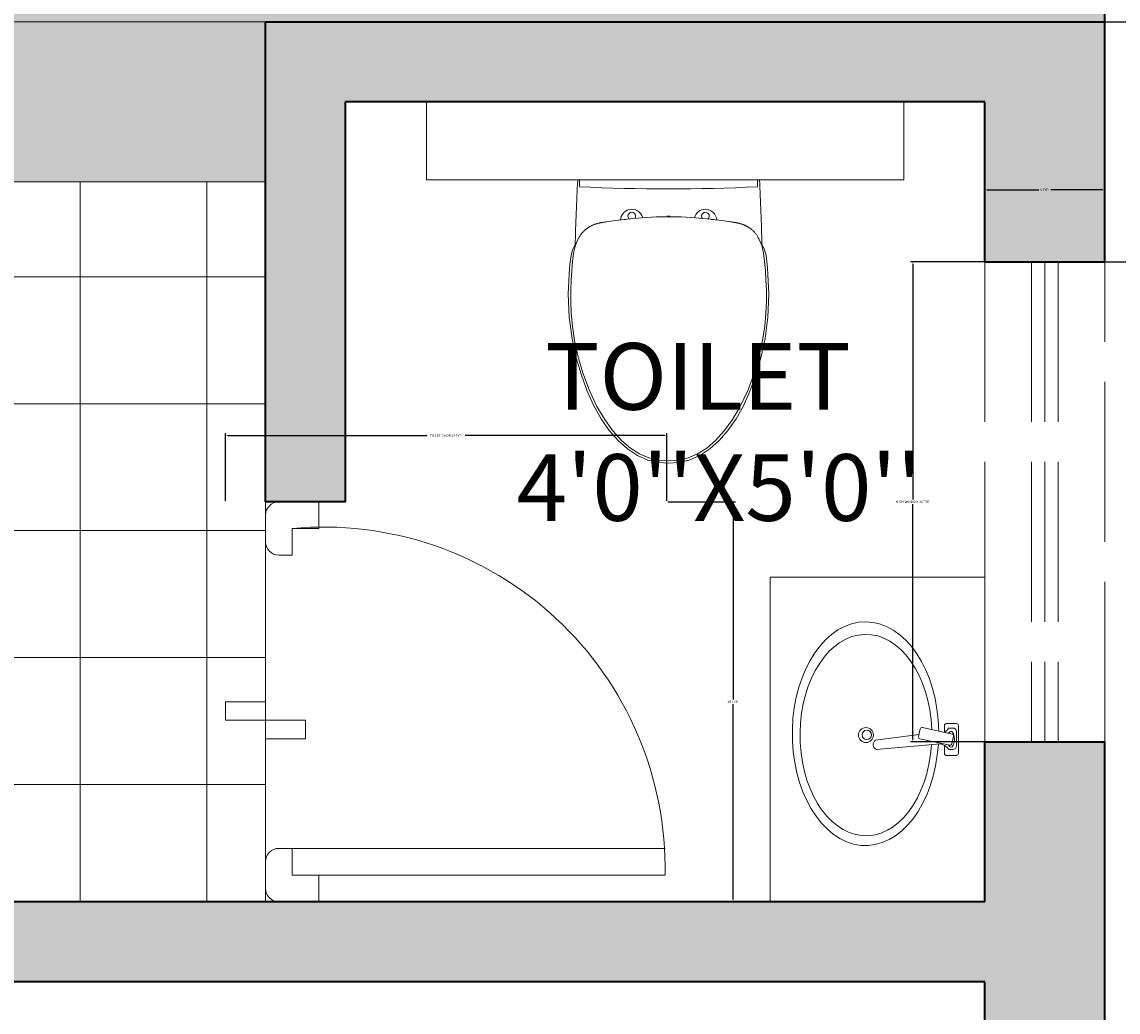
# Model space of a CAD drawing. Units: inches. Extents: x 84 to 1044, y -280 to 906.
# Tile 80 of 105: x 815 to 897, y 326 to 400. Entities that reach past the tile are written whole.
import ezdxf

# ---------------------------------------------------------------- set-up
doc = ezdxf.new("R2010")
doc.units = ezdxf.units.IN
doc.linetypes.add('ACAD_ISO02W100', pattern=[15, 12, -3])
for name, color, linetype, lineweight in [('00 FURNITURE', 15, 'Continuous', 15), ('A-ANNO-DIMS', 2, 'Continuous', 18), ('A-AREA-IDEN', 7, 'Continuous', 13), ('A-DOOR', 4, 'Continuous', 18), ('A-FLOR-FIXT', 9, 'Continuous', 15), ('A-GLAZ-HIGH', 160, 'ACAD_ISO02W100', 13), ('A-STAIRCASE', 144, 'Continuous', 18), ('A_FUR 1', 5, 'Continuous', 5), ('WALL', 250, 'Continuous', 35)]:
    doc.layers.add(name, color=color, linetype=linetype, lineweight=lineweight)
for name, color, linetype, lineweight, true_color in [('A-FLOR-PATT', 251, 'Continuous', 9, 0x705861), ('A-FLOR-STRS-PATT', 35, 'Continuous', 9, 0x947764), ('A-WALL-PATT', 251, 'Continuous', 9, 0x636466), ('L-PLNT-PATT', 9, 'Continuous', 9, 0xafd9aa)]:
    doc.layers.add(name, color=color, linetype=linetype, lineweight=lineweight, true_color=true_color)
doc.styles.add('1-100DIM', font='txt', dxfattribs={"height": 0.3})
doc.styles.get("Standard").update_dxf_attribs({"font": 'arial.ttf'})
doc.dimstyles.get("Standard").update_dxf_attribs({"dimtxt": 0.18, "dimasz": 0.18, "dimexe": 0.18, "dimexo": 0.0625, "dimgap": 0.09, "dimtad": 0, "dimtih": 1, "dimtoh": 1, "dimdec": 4, "dimzin": 0, "dimdsep": 46, "dimtxsty": 'Standard', "dimcen": 0.09, "dimadec": 0, "dimazin": 0, "dimtfac": 1, "dimtdec": 4, "dimtofl": 0, "dimtmove": 0, "dimatfit": 3, "dimfxl": 1, "dimtolj": 1, "dimtzin": 0, "dimarcsym": 0})

# ---------------------------------------------------------------- blocks, each defined once
blk = doc.blocks.new('ESTSET')
at = {"layer": 'A_FUR 1'}
for p, q in [((-10.444, 4.097), (-10.444, 32.097)), ((-8.444, 4.097), (-8.444, 32.097)), ((-36.444, 6.097), (-36.444, 3.097)), ((-34.444, 6.097), (-36.444, 6.097)), ((-34.444, 4.097), (-34.444, 6.097)), ((-34.444, 4.097), (-34.444, 6.097)), ((-8.444, 4.097), (-8.444, 6.097)), ((-8.444, 6.097), (-6.444, 6.097)), ((-8.444, 4.097), (-8.444, 6.097)), ((-6.444, 6.097), (-6.444, 3.097)), ((-32.444, 4.097), (-34.444, 4.097)), ((-32.444, 4.097), (-34.444, 4.097)), ((-32.444, 3.097), (-32.444, 4.097)), ((-10.444, 3.097), (-10.444, 4.097)), ((-10.444, 4.097), (-8.444, 4.097)), ((-10.444, 4.097), (-8.444, 4.097)), ((-6.444, 2.097), (-36.444, 2.097)), ((-35.444, 2.097), (-33.444, 2.097)), ((-7.444, 2.097), (-9.444, 2.097))]:
    blk.add_line(p, q, dxfattribs=at)
for points in [[(-21.444, 2.097), (-18.672, 2.097), (-18.672, 5.102), (-20.058, 5.102)], [(-20.058, 5.102), (-20.058, -0.909)], [(-21.444, 2.097), (-21.444, -0.909), (-20.058, -0.909)]]:
    blk.add_lwpolyline(points, dxfattribs=at)
for centre, radius, start, end in [((-8.909, 6.457), 25.644, 88.96059, 185.2816), ((-35.444, 3.097), 1, 180, 270), ((-33.444, 3.097), 1, 270, 0), ((-9.444, 3.097), 1, 180, 270), ((-7.444, 3.097), 1, 270, 0)]:
    blk.add_arc(centre, radius, start, end, dxfattribs=at)
blk = doc.blocks.new('32')
at = {"layer": '00 FURNITURE'}
for p, q in [((-6.823, 0), (6.823, 0)), ((-6.685, -0.511), (-6.685, 0)), ((6.237, 0), (6.685, 0)), ((6.685, -0.511), (6.685, 0)), ((-5.414, -3.288), (-5.444, -3.297)), ((-5.385, -3.279), (-5.414, -3.288)), ((-5.356, -3.271), (-5.385, -3.279)), ((-5.328, -3.264), (-5.356, -3.271)), ((-5.301, -3.256), (-5.328, -3.264)), ((-5.273, -3.249), (-5.301, -3.256)), ((-5.247, -3.242), (-5.273, -3.249)), ((-5.22, -3.236), (-5.247, -3.242)), ((-5.195, -3.23), (-5.22, -3.236)), ((-5.17, -3.225), (-5.195, -3.23)), ((-5.145, -3.219), (-5.17, -3.225)), ((-5.121, -3.214), (-5.145, -3.219)), ((-5.098, -3.209), (-5.121, -3.214)), ((-5.076, -3.205), (-5.098, -3.209)), ((-5.053, -3.2), (-5.076, -3.205)), ((-5.032, -3.196), (-5.053, -3.2)), ((-5.011, -3.193), (-5.032, -3.196)), ((-4.97, -3.185), (-5.011, -3.193)), ((-4.931, -3.179), (-4.97, -3.185)), ((-4.893, -3.173), (-4.931, -3.179)), ((-4.858, -3.167), (-4.893, -3.173)), ((-4.824, -3.162), (-4.858, -3.167)), ((-4.776, -3.155), (-4.824, -3.162)), ((-4.717, -3.147), (-4.776, -3.155)), ((-4.627, -3.135), (-4.717, -3.147)), ((-4.464, -3.111), (-4.637, -3.136)), ((-4.345, -3.095), (-4.464, -3.111)), ((-4.151, -3.069), (-4.345, -3.095)), ((-3.99, -3.048), (-4.151, -3.069)), ((-3.77, -3.021), (-3.99, -3.048)), ((-3.503, -2.989), (-3.77, -3.021)), ((-3.335, -2.969), (-3.503, -2.989)), ((-3.3, -2.966), (-3.32, -2.968)), ((-3.257, -2.962), (-3.3, -2.966)), ((-3.212, -2.958), (-3.257, -2.962)), ((-3.146, -2.951), (-3.205, -2.957)), ((-2.011, -2.841), (-3.146, -2.951)), ((-0.935, -2.777), (-2.011, -2.841)), ((0, -2.757), (-0.935, -2.777)), ((0.118, -2.713), (-0.118, -2.713)), ((0, -2.757), (0.935, -2.777)), ((0.935, -2.777), (2.011, -2.841)), ((2.011, -2.841), (3.146, -2.951)), ((3.146, -2.951), (3.205, -2.957)), ((3.212, -2.958), (3.257, -2.962)), ((3.257, -2.962), (3.3, -2.966)), ((3.3, -2.966), (3.32, -2.968)), ((3.335, -2.969), (3.503, -2.989)), ((3.503, -2.989), (3.77, -3.021)), ((3.77, -3.021), (3.99, -3.048)), ((3.99, -3.048), (4.151, -3.069)), ((4.151, -3.069), (4.345, -3.095)), ((4.345, -3.095), (4.464, -3.111)), ((4.464, -3.111), (4.637, -3.136)), ((4.627, -3.135), (4.717, -3.147)), ((4.717, -3.147), (4.776, -3.155)), ((4.776, -3.155), (4.824, -3.162)), ((4.824, -3.162), (4.858, -3.167)), ((4.858, -3.167), (4.893, -3.173)), ((4.893, -3.173), (4.931, -3.179)), ((4.931, -3.179), (4.97, -3.185)), ((4.97, -3.185), (5.011, -3.193)), ((5.011, -3.193), (5.032, -3.196)), ((5.032, -3.196), (5.053, -3.2)), ((5.053, -3.2), (5.076, -3.205)), ((5.076, -3.205), (5.098, -3.209)), ((5.098, -3.209), (5.121, -3.214)), ((5.121, -3.214), (5.145, -3.219)), ((5.145, -3.219), (5.17, -3.225)), ((5.17, -3.225), (5.195, -3.23)), ((5.195, -3.23), (5.22, -3.236)), ((5.22, -3.236), (5.247, -3.242)), ((5.247, -3.242), (5.273, -3.249)), ((5.273, -3.249), (5.301, -3.256)), ((5.301, -3.256), (5.328, -3.264)), ((5.328, -3.264), (5.356, -3.271)), ((5.356, -3.271), (5.385, -3.279)), ((5.385, -3.279), (5.414, -3.288)), ((5.414, -3.288), (5.444, -3.297)), ((-6.579, -4.082), (-6.611, -4.127)), ((-6.547, -4.039), (-6.579, -4.082)), ((-6.514, -3.997), (-6.547, -4.039)), ((-6.481, -3.958), (-6.514, -3.997)), ((-6.447, -3.92), (-6.481, -3.958)), ((-6.413, -3.882), (-6.447, -3.92)), ((-6.378, -3.847), (-6.413, -3.882)), ((-6.343, -3.813), (-6.378, -3.847)), ((-6.307, -3.779), (-6.343, -3.813)), ((-6.271, -3.748), (-6.307, -3.779)), ((-6.235, -3.717), (-6.271, -3.748)), ((-6.199, -3.687), (-6.235, -3.717)), ((-6.162, -3.659), (-6.199, -3.687)), ((-6.125, -3.632), (-6.162, -3.659)), ((-6.088, -3.606), (-6.125, -3.632)), ((-6.052, -3.581), (-6.088, -3.606)), ((-6.015, -3.557), (-6.052, -3.581)), ((-5.978, -3.535), (-6.015, -3.557)), ((-5.942, -3.513), (-5.978, -3.535)), ((-5.906, -3.493), (-5.942, -3.513)), ((-5.869, -3.473), (-5.906, -3.493)), ((-5.834, -3.455), (-5.869, -3.473)), ((-5.798, -3.437), (-5.834, -3.455)), ((-5.763, -3.421), (-5.798, -3.437)), ((-5.729, -3.405), (-5.763, -3.421)), ((-5.695, -3.39), (-5.729, -3.405)), ((-5.662, -3.376), (-5.695, -3.39)), ((-5.629, -3.363), (-5.662, -3.376)), ((-5.597, -3.351), (-5.629, -3.363)), ((-5.565, -3.339), (-5.597, -3.351)), ((-5.534, -3.328), (-5.565, -3.339)), ((-5.504, -3.317), (-5.534, -3.328)), ((-5.474, -3.307), (-5.504, -3.317)), ((-5.444, -3.297), (-5.474, -3.307)), ((5.444, -3.297), (5.474, -3.307)), ((5.474, -3.307), (5.504, -3.317)), ((5.504, -3.317), (5.534, -3.328)), ((5.534, -3.328), (5.565, -3.339)), ((5.565, -3.339), (5.597, -3.351)), ((5.597, -3.351), (5.629, -3.363)), ((5.629, -3.363), (5.662, -3.376)), ((5.662, -3.376), (5.695, -3.39)), ((5.695, -3.39), (5.729, -3.405)), ((5.729, -3.405), (5.763, -3.421)), ((5.763, -3.421), (5.798, -3.437)), ((5.798, -3.437), (5.834, -3.455)), ((5.834, -3.455), (5.869, -3.473)), ((5.869, -3.473), (5.906, -3.493)), ((5.906, -3.493), (5.942, -3.513)), ((5.942, -3.513), (5.978, -3.535)), ((5.978, -3.535), (6.015, -3.557)), ((6.015, -3.557), (6.052, -3.581)), ((6.052, -3.581), (6.088, -3.606)), ((6.088, -3.606), (6.125, -3.632)), ((6.125, -3.632), (6.162, -3.659)), ((6.162, -3.659), (6.199, -3.687)), ((6.199, -3.687), (6.235, -3.717)), ((6.235, -3.717), (6.271, -3.748)), ((6.271, -3.748), (6.307, -3.779)), ((6.307, -3.779), (6.343, -3.813)), ((6.343, -3.813), (6.378, -3.847)), ((6.378, -3.847), (6.413, -3.882)), ((6.413, -3.882), (6.447, -3.92)), ((6.447, -3.92), (6.481, -3.958)), ((6.481, -3.958), (6.514, -3.997)), ((6.514, -3.997), (6.547, -4.039)), ((6.547, -4.039), (6.579, -4.082)), ((6.579, -4.082), (6.611, -4.127)), ((-7.013, -4.856), (-7.206, -5.236)), ((-6.992, -4.903), (-7.128, -5.488)), ((-6.93, -4.757), (-7.013, -4.856)), ((-6.786, -4.418), (-6.992, -4.903)), ((-6.769, -4.387), (-6.786, -4.418)), ((-6.736, -4.329), (-6.769, -4.387)), ((-6.705, -4.275), (-6.736, -4.329)), ((-6.674, -4.223), (-6.705, -4.275)), ((-6.642, -4.174), (-6.674, -4.223)), ((-6.611, -4.127), (-6.642, -4.174)), ((6.611, -4.127), (6.643, -4.174)), ((6.643, -4.174), (6.674, -4.223)), ((6.674, -4.223), (6.705, -4.275)), ((6.705, -4.275), (6.736, -4.329)), ((6.736, -4.329), (6.769, -4.387)), ((6.769, -4.387), (6.786, -4.418)), ((6.786, -4.418), (6.992, -4.903)), ((6.93, -4.757), (7.013, -4.856)), ((6.992, -4.903), (7.128, -5.488)), ((7.013, -4.856), (7.206, -5.236)), ((-7.32, -5.673), (-7.386, -6.148)), ((-7.206, -5.236), (-7.32, -5.673)), ((-7.128, -5.488), (-7.208, -6.118)), ((7.128, -5.488), (7.208, -6.118)), ((7.206, -5.236), (7.32, -5.673)), ((7.32, -5.673), (7.386, -6.148)), ((-7.386, -6.148), (-7.435, -6.616)), ((-7.208, -6.118), (-7.266, -6.79)), ((7.208, -6.118), (7.266, -6.79)), ((7.386, -6.148), (7.435, -6.616)), ((-7.436, -6.626), (-7.53, -8.534)), ((-7.266, -6.79), (-7.311, -7.508)), ((7.266, -6.79), (7.311, -7.508)), ((7.436, -6.626), (7.53, -8.534)), ((-7.311, -7.508), (-7.338, -8.278)), ((7.311, -7.508), (7.338, -8.278)), ((-7.53, -8.534), (-7.452, -10.295)), ((-7.338, -8.278), (-7.338, -9.106)), ((7.338, -8.278), (7.338, -9.106)), ((7.53, -8.534), (7.452, -10.295)), ((-7.338, -9.106), (-7.301, -10.001)), ((7.338, -9.106), (7.301, -10.001)), ((-7.452, -10.295), (-7.242, -11.89)), ((-7.301, -10.001), (-7.213, -10.974)), ((7.301, -10.001), (7.214, -10.974)), ((7.452, -10.295), (7.242, -11.89)), ((-7.213, -10.974), (-7.057, -12.031)), ((7.214, -10.974), (7.057, -12.031)), ((-7.242, -11.89), (-6.932, -13.338)), ((-7.057, -12.031), (-6.809, -13.187)), ((7.057, -12.031), (6.809, -13.187)), ((7.242, -11.89), (6.932, -13.338)), ((-6.932, -13.338), (-6.548, -14.655)), ((-6.809, -13.187), (-6.438, -14.479)), ((6.809, -13.187), (6.438, -14.479)), ((6.932, -13.338), (6.548, -14.655)), ((-6.548, -14.655), (-6.109, -15.853)), ((-6.438, -14.479), (-5.945, -15.803)), ((6.438, -14.479), (5.945, -15.803)), ((6.548, -14.655), (6.109, -15.853)), ((-6.109, -15.853), (-5.615, -16.941)), ((-5.945, -15.803), (-5.384, -16.987)), ((5.945, -15.803), (5.384, -16.987)), ((6.109, -15.853), (5.615, -16.941)), ((-5.615, -16.941), (-5.063, -17.918)), ((-5.384, -16.987), (-4.794, -17.979)), ((5.384, -16.987), (4.794, -17.979)), ((5.615, -16.941), (5.063, -17.918)), ((-5.063, -17.918), (-4.455, -18.783)), ((-4.794, -17.979), (-4.173, -18.826)), ((4.794, -17.979), (4.173, -18.826)), ((5.063, -17.918), (4.455, -18.783)), ((-4.455, -18.783), (-3.795, -19.536)), ((-4.173, -18.826), (-3.529, -19.539)), ((4.173, -18.826), (3.529, -19.539)), ((4.455, -18.783), (3.795, -19.536)), ((-3.795, -19.536), (-3.09, -20.171)), ((-3.529, -19.539), (-2.863, -20.116)), ((3.529, -19.539), (2.863, -20.116)), ((3.795, -19.536), (3.09, -20.171)), ((-3.09, -20.171), (-2.339, -20.67)), ((-2.863, -20.116), (-2.179, -20.552)), ((-2.179, -20.552), (-1.472, -20.853)), ((2.179, -20.552), (1.472, -20.853)), ((2.863, -20.116), (2.179, -20.552)), ((3.09, -20.171), (2.339, -20.67)), ((-2.339, -20.67), (-1.549, -21.013)), ((-1.549, -21.013), (-0.748, -21.198)), ((-1.472, -20.853), (-0.736, -21.027)), ((-0.748, -21.198), (0, -21.25)), ((-0.736, -21.027), (0, -21.082)), ((0.736, -21.027), (0, -21.082)), ((0.748, -21.198), (0, -21.25)), ((1.472, -20.853), (0.736, -21.027)), ((1.549, -21.013), (0.748, -21.198)), ((2.339, -20.67), (1.549, -21.013))]:
    blk.add_line(p, q, dxfattribs=at)
for points in [[(-6.823, 0), (-6.906, -1.63), (-6.969, -3.262), (-7.011, -4.894)], [(7.011, -4.894), (6.969, -3.262), (6.906, -1.63), (6.823, 0)], [(-6.685, -0.511), (-2.231, -0.73), (2.231, -0.73), (6.685, -0.511)], [(-2.974, -2.227), (-3.332, -2.32), (-3.589, -2.633), (-3.609, -3.001)], [(-1.941, -2.837), (-2.058, -2.383), (-2.52, -2.11), (-2.974, -2.227)], [(-2.583, -2.49), (-2.634, -2.449), (-2.697, -2.427), (-2.762, -2.427)], [(2.762, -2.2), (2.375, -2.2), (2.037, -2.462), (1.941, -2.837)], [(3.609, -3.001), (3.584, -2.552), (3.212, -2.2), (2.762, -2.2)], [(2.98, -2.528), (2.926, -2.464), (2.846, -2.427), (2.762, -2.427)], [(-2.539, -2.892), (-2.44, -2.769), (-2.46, -2.589), (-2.583, -2.49)], [(2.947, -2.932), (3.067, -2.829), (3.082, -2.649), (2.98, -2.528)]]:
    blk.add_open_spline(points, degree=3, dxfattribs=at)
for points in [[(-2.762, -2.427), (-2.92, -2.427), (-3.048, -2.555), (-3.048, -2.713), (-3.048, -2.797), (-3.011, -2.877), (-2.947, -2.932)], [(2.762, -2.427), (2.604, -2.427), (2.476, -2.555), (2.476, -2.713), (2.476, -2.778), (2.498, -2.841), (2.539, -2.892)]]:
    blk.add_open_spline(points, degree=3, knots=[0, 0, 0, 0, 1, 1, 1, 2, 2, 2, 2], dxfattribs=at)
blk = doc.blocks.new('WWCC')
at = {"layer": '00 FURNITURE', "ltscale": 20}
blk.add_lwpolyline([(140241.579, -48678.243), (140247.434, -48678.243), (140247.434, -48714.064), (140241.579, -48714.064)], close=True, dxfattribs=at)
at = {"layer": '00 FURNITURE', "rotation": 90.00000000000003}
blk.add_blockref('32', (140247.434, -48695.892), dxfattribs=at)
blk = doc.blocks.new('WIN-HIGH-36IN')
for p, q in [((3.499, 36), (3.499, 0)), ((4.499, 36), (4.499, 0)), ((5.499, 36), (5.499, 0))]:
    blk.add_line(p, q)
blk.add_lwpolyline([(-0.001, 0), (8.999, 0), (8.999, 36), (-0.001, 36)], close=True)
blk = doc.blocks.new('*D36')
at = {"layer": 'A-ANNO-DIMS', "color": 0, "lineweight": -2, "transparency": 16777216}
for p, q in [((887.011, 382.12), (881.494, 382.12)), ((881.674, 381.94), (881.674, 364.303)), ((881.674, 346.3), (881.674, 363.937)), ((887.011, 346.12), (881.494, 346.12))]:
    blk.add_line(p, q, dxfattribs=at)
at = {"layer": 'A-ANNO-DIMS', "color": 0, "transparency": 16777216}
for points in [[(881.644, 381.94), (881.704, 381.94), (881.674, 382.12)], [(881.644, 346.3), (881.704, 346.3), (881.674, 346.12)]]:
    blk.add_solid(points, dxfattribs=at)
at = {"layer": 'Defpoints', "color": 0, "transparency": 16777216}
for p in [(881.674, 382.12), (887.074, 382.12), (887.074, 346.12)]:
    blk.add_point(p, dxfattribs=at)
at = {"layer": 'A-ANNO-DIMS', "color": 0, "transparency": 16777216, "insert": (881.674, 364.12), "char_height": 0.18, "attachment_point": 5}
blk.add_mtext('\\A1;HIGH WINDOW 36 TYP.', dxfattribs=at)
blk = doc.blocks.new('*D37')
at = {"layer": 'A-ANNO-DIMS', "color": 0, "lineweight": -2, "transparency": 16777216}
for p, q in [((887.074, 382.183), (887.074, 387.7)), ((896.074, 382.183), (896.074, 387.7)), ((887.254, 387.52), (891.116, 387.52)), ((895.894, 387.52), (892.032, 387.52))]:
    blk.add_line(p, q, dxfattribs=at)
at = {"layer": 'A-ANNO-DIMS', "color": 0, "transparency": 16777216}
for points in [[(887.254, 387.55), (887.254, 387.49), (887.074, 387.52)], [(895.894, 387.55), (895.894, 387.49), (896.074, 387.52)]]:
    blk.add_solid(points, dxfattribs=at)
at = {"layer": 'Defpoints', "color": 0, "transparency": 16777216}
for p in [(896.074, 387.52), (887.074, 382.12), (896.074, 382.12)]:
    blk.add_point(p, dxfattribs=at)
at = {"layer": 'A-ANNO-DIMS', "color": 0, "transparency": 16777216, "insert": (891.574, 387.52), "char_height": 0.18, "attachment_point": 5}
blk.add_mtext('\\A1;9 TYP.', dxfattribs=at)
blk = doc.blocks.new('*D40')
at = {"layer": 'A-ANNO-DIMS', "color": 0, "lineweight": -2, "transparency": 16777216}
for p, q in [((830.069, 364.183), (830.069, 369.271)), ((830.249, 369.091), (845.22, 369.091)), ((863.026, 369.091), (848.055, 369.091)), ((863.206, 364.183), (863.206, 369.271))]:
    blk.add_line(p, q, dxfattribs=at)
at = {"layer": 'A-ANNO-DIMS', "color": 0, "transparency": 16777216}
for points in [[(830.249, 369.121), (830.249, 369.061), (830.069, 369.091)], [(863.026, 369.121), (863.026, 369.061), (863.206, 369.091)]]:
    blk.add_solid(points, dxfattribs=at)
at = {"layer": 'Defpoints', "color": 0, "transparency": 16777216}
for p in [(863.206, 369.091), (830.069, 364.12), (863.206, 364.12)]:
    blk.add_point(p, dxfattribs=at)
at = {"layer": 'A-ANNO-DIMS', "color": 0, "transparency": 16777216, "insert": (846.637, 369.091), "char_height": 0.18, "attachment_point": 5}
blk.add_mtext('\\A1;TOILET DOOR 33 TYP.', dxfattribs=at)
blk = doc.blocks.new('*D41')
at = {"layer": 'A-ANNO-DIMS', "color": 0, "lineweight": -2, "transparency": 16777216}
for p, q in [((863.269, 364.12), (868.357, 364.12)), ((868.177, 363.94), (868.177, 349.302)), ((868.177, 334.3), (868.177, 348.938)), ((863.269, 334.12), (868.357, 334.12))]:
    blk.add_line(p, q, dxfattribs=at)
at = {"layer": 'A-ANNO-DIMS', "color": 0, "transparency": 16777216}
for points in [[(868.147, 363.94), (868.207, 363.94), (868.177, 364.12)], [(868.147, 334.3), (868.207, 334.3), (868.177, 334.12)]]:
    blk.add_solid(points, dxfattribs=at)
at = {"layer": 'Defpoints', "color": 0, "transparency": 16777216}
for p in [(863.206, 364.12), (863.206, 334.12), (868.177, 334.12)]:
    blk.add_point(p, dxfattribs=at)
at = {"layer": 'A-ANNO-DIMS', "color": 0, "transparency": 16777216, "insert": (868.177, 349.12), "char_height": 0.18, "attachment_point": 5}
blk.add_mtext('\\A1;30 TYP.', dxfattribs=at)
blk = doc.blocks.new('*D63')
at = {"layer": 'A-ANNO-DIMS', "color": 0, "lineweight": -2, "transparency": 16777216}
for p, q in [((833.136, 709.12), (1043.768, 709.12)), ((1043.588, 708.94), (1043.588, 400.302)), ((1043.588, 91.3), (1043.588, 399.938)), ((896.136, 91.12), (1043.768, 91.12))]:
    blk.add_line(p, q, dxfattribs=at)
at = {"layer": 'A-ANNO-DIMS', "color": 0, "transparency": 16777216}
for points in [[(1043.558, 708.94), (1043.618, 708.94), (1043.588, 709.12)], [(1043.558, 91.3), (1043.618, 91.3), (1043.588, 91.12)]]:
    blk.add_solid(points, dxfattribs=at)
at = {"layer": 'Defpoints', "color": 0, "transparency": 16777216}
for p in [(833.074, 709.12), (1043.588, 709.12), (896.074, 91.12)]:
    blk.add_point(p, dxfattribs=at)
at = {"layer": 'A-ANNO-DIMS', "color": 0, "transparency": 16777216, "insert": (1043.588, 400.12), "char_height": 0.18, "attachment_point": 5}
blk.add_mtext('\\A1;618', dxfattribs=at)
blk = doc.blocks.new('*D76')
at = {"layer": 'A-ANNO-DIMS', "color": 0, "lineweight": -2, "transparency": 16777216}
for p, q in [((896.136, 400.12), (1043.768, 400.12)), ((1043.588, 399.94), (1043.588, 391.302)), ((1043.588, 382.3), (1043.588, 390.938)), ((896.136, 382.12), (1043.768, 382.12))]:
    blk.add_line(p, q, dxfattribs=at)
at = {"layer": 'A-ANNO-DIMS', "color": 0, "transparency": 16777216}
for points in [[(1043.558, 399.94), (1043.618, 399.94), (1043.588, 400.12)], [(1043.558, 382.3), (1043.618, 382.3), (1043.588, 382.12)]]:
    blk.add_solid(points, dxfattribs=at)
at = {"layer": 'Defpoints', "color": 0, "transparency": 16777216}
for p in [(896.074, 400.12), (1043.588, 400.12), (896.074, 382.12)]:
    blk.add_point(p, dxfattribs=at)
at = {"layer": 'A-ANNO-DIMS', "color": 0, "transparency": 16777216, "insert": (1043.588, 391.12), "char_height": 0.18, "attachment_point": 5}
blk.add_mtext('\\A1;18', dxfattribs=at)

msp = doc.modelspace()

# ---------------------------------------------------------------- hatches: boundary and pattern name
at = {"layer": 'A-FLOR-PATT', "transparency": 33554597}
h = msp.add_hatch(dxfattribs=at)
h.set_pattern_fill('ANSI37', color=256, scale=3, angle=45)
h.paths.add_polyline_path([(833.074, 388.12), (704.074, 388.12), (704.074, 370.12), (695.074, 370.12), (695.074, 334.12), (732.574, 334.12), (804.574, 334.12), (833.074, 334.12), (833.074, 364.12)])
at = {"layer": 'A-FLOR-STRS-PATT', "transparency": 33554567}
h = msp.add_hatch(color=256, dxfattribs=at)
h.dxf.hatch_style = 1
h.paths.add_polyline_path([(833.074, 400.12), (704.074, 400.12), (704.074, 388.12), (833.074, 388.12)])
at = {"layer": 'A-WALL-PATT', "transparency": 33554597}
h = msp.add_hatch(color=256, dxfattribs=at)
h.dxf.hatch_style = 1
h.paths.add_polyline_path([(671.074, 100.12), (647.074, 100.12), (647.074, 160.12), (641.074, 160.12), (620.824, 160.12), (620.824, 151.12), (638.074, 151.12), (638.074, 91.12), (671.074, 91.12)])
h.paths.add_polyline_path([(791.074, 100.12), (743.074, 100.12), (743.074, 91.12), (791.074, 91.12)])
h.paths.add_polyline_path([(896.074, 346.12), (887.074, 346.12), (887.074, 334.12), (870.955, 334.12), (833.074, 334.12), (804.574, 334.12), (804.574, 328.12), (887.074, 328.12), (887.074, 100.12), (863.074, 100.12), (863.074, 91.12), (896.074, 91.12)])
h.paths.add_polyline_path([(507.574, 154.729), (507.574, 160.12), (464.074, 160.12), (464.074, 247.12), (641.074, 247.12), (641.074, 208.12), (647.074, 208.12), (647.074, 328.12), (659.074, 328.12), (659.074, 334.12), (617.074, 334.12), (617.074, 328.12), (641.074, 328.12), (641.074, 256.12), (545.074, 256.12), (545.074, 328.12), (569.074, 328.12), (569.074, 334.12), (518.074, 334.12), (518.074, 325.12), (536.074, 325.12), (536.074, 256.12), (464.074, 256.12), (464.074, 325.12), (482.074, 325.12), (482.074, 334.12), (455.074, 334.12), (455.074, 160.12), (413.127, 160.12), (413.127, 151.12), (455.074, 151.12), (455.074, 91.12), (464.074, 91.12), (464.074, 151.12), (507.574, 151.12)])
h.paths.add_polyline_path([(572.824, 160.12), (555.574, 160.12), (555.574, 151.12), (572.824, 151.12)], flags=17)
h.paths.add_polyline_path([(341.127, 160.12), (299.179, 160.12), (299.179, 211.12), (294.179, 211.12), (290.179, 211.12), (290.179, 151.12), (341.127, 151.12)])
h.paths.add_polyline_path([(299.179, 256.12), (212.179, 256.12), (212.179, 274.12), (203.179, 274.12), (203.179, 247.12), (299.179, 247.12)])
h.paths.add_polyline_path([(212.179, 514.12), (398.074, 514.12), (398.074, 519.12), (398.074, 520.12), (212.179, 520.12), (212.179, 574.12), (203.179, 574.12), (203.179, 310.12), (212.179, 310.12), (212.179, 328.12), (290.179, 328.12), (290.179, 292.12), (299.179, 292.12), (299.179, 328.12), (332.179, 328.12), (332.179, 334.12), (212.179, 334.12)])
h.paths.add_polyline_path([(287.127, 709.12), (203.179, 709.12), (203.179, 646.12), (212.179, 646.12), (212.179, 700.12), (287.127, 700.12)])
h.paths.add_polyline_path([(470.074, 709.12), (359.127, 709.12), (359.127, 700.12), (434.074, 700.12), (434.074, 574.12), (440.074, 574.12), (440.074, 622.12), (464.074, 622.12), (464.074, 628.12), (440.074, 628.12), (440.074, 700.12), (470.074, 700.12)])
h.paths.add_polyline_path([(572.074, 709.12), (506.074, 709.12), (506.074, 700.12), (536.074, 700.12), (536.074, 628.12), (494.074, 628.12), (494.074, 622.12), (536.074, 622.12), (536.074, 520.12), (440.074, 520.12), (440.074, 544.12), (434.074, 544.12), (434.074, 514.12), (644.074, 514.12), (644.074, 519.12), (644.074, 544.12), (638.074, 544.12), (638.074, 520.12), (542.074, 520.12), (542.074, 622.12), (584.074, 622.12), (584.074, 628.12), (542.074, 628.12), (542.074, 700.12), (572.074, 700.12)])
h.paths.add_polyline_path([(698.074, 709.12), (608.074, 709.12), (608.074, 700.12), (638.074, 700.12), (638.074, 628.12), (614.074, 628.12), (614.074, 622.12), (638.074, 622.12), (638.074, 574.12), (644.074, 574.12), (644.074, 700.12), (698.074, 700.12)])
h.paths.add_polyline_path([(833.074, 709.12), (770.074, 709.12), (770.074, 700.12), (824.074, 700.12), (824.074, 646.12), (833.074, 646.12)])
h.paths.add_polyline_path([(833.074, 574.12), (824.074, 574.12), (824.074, 520.12), (791.244, 520.12), (712.904, 520.12), (680.074, 520.12), (680.074, 514.12), (695.074, 514.12), (695.074, 491.62), (704.074, 491.62), (704.074, 511.12), (833.074, 511.12)])
h.paths.add_polyline_path([(704.074, 419.62), (695.074, 419.62), (695.074, 370.12), (704.074, 370.12)])
h.paths.add_polyline_path([(896.074, 400.12), (833.074, 400.12), (833.074, 364.12), (839.074, 364.12), (839.074, 394.12), (887.074, 394.12), (887.074, 382.12), (896.074, 382.12)])
h.paths.add_polyline_path([(732.574, 334.12), (695.074, 334.12), (695.074, 328.12), (732.574, 328.12)])
at = {"layer": 'L-PLNT-PATT', "transparency": 33554597}
h = msp.add_hatch(color=256, dxfattribs=at)
h.dxf.hatch_style = 1
h.paths.add_polyline_path([(896.074, 511.12), (704.074, 511.12), (704.074, 491.62), (704.074, 419.62), (704.074, 400.12), (833.074, 400.12), (896.074, 400.12)])

# ---------------------------------------------------------------- linework, layer by layer
at = {"layer": 'A-DOOR'}
msp.add_line((833.074, 364.12), (833.074, 334.12), dxfattribs=at)
at = {"layer": 'A-FLOR-FIXT'}
for p, q in [((870.955, 334.12), (870.955, 358.462)), ((870.955, 358.462), (887.074, 358.462)), ((887.074, 358.462), (887.074, 334.12)), ((882.133, 346.664), (878.878, 346.251)), ((884.672, 347.149), (884.355, 347.149)), ((884.942, 345.815), (884.942, 346.879)), ((883.732, 345.956), (878.95, 345.542)), ((884.672, 345.545), (884.373, 345.545)), ((870.955, 334.12), (887.074, 334.12))]:
    msp.add_line(p, q, dxfattribs=at)
msp.add_lwpolyline([(884.046, 346.823), (884.046, 347.349, -0.414214), (884.181, 347.485), (884.956, 347.485, -0.414214), (885.091, 347.349), (885.091, 345.233, -0.414214), (884.956, 345.098), (884.181, 345.098, -0.414214), (884.046, 345.233), (884.046, 345.832)], format="xyb", dxfattribs=at)
msp.add_lwpolyline([(884.437, 345.864), (882.203, 346.349, -0.414214), (882.1, 346.51), (882.224, 347.082, -0.414214), (882.385, 347.185), (884.619, 346.699, -0.414214), (884.722, 346.538), (884.598, 345.967, -0.414214)], format="xyb", close=True, dxfattribs=at)
for centre, radius in [((878.146, 346.623), 0.558), ((878.146, 346.623), 0.558), ((878.214, 346.632), 0.351)]:
    msp.add_circle(centre, radius, dxfattribs=at)
for centre, radius, start, end in [((883.412, 347.752), 1.12, 304.12446, 327.43003), ((884.672, 346.879), 0.27, 0, 90), ((879.091, 345.914), 0.398, 122.34148, 249.24278), ((883.485, 344.864), 1.12, 37.5091, 77.23745), ((884.672, 345.815), 0.27, 270, 0)]:
    msp.add_arc(centre, radius, start, end, dxfattribs=at)
for centre, major_axis, ratio, start_param, end_param in [((878.115, 346.727), (0, 8.396), 0.654321, -1.54793, 4.618862), ((878.146, 346.623), (0, 7.556), 0.654321, -1.516557, 4.61628), ((884.525, 346.304), (0, -0.599), 0.443478, -0.799654, 3.854588)]:
    msp.add_ellipse(centre, major_axis=major_axis, ratio=ratio, start_param=start_param, end_param=end_param, dxfattribs=at)
at = {"layer": 'A-STAIRCASE'}
for p, q in [((833.074, 400.12), (704.074, 400.12)), ((833.074, 388.12), (704.074, 388.12))]:
    msp.add_line(p, q, dxfattribs=at)
at = {"layer": 'WALL'}
for p, q in [((896.074, 400.12), (896.074, 511.12)), ((833.074, 364.12), (833.074, 400.12)), ((833.074, 400.12), (896.074, 400.12)), ((896.074, 382.12), (896.074, 400.12)), ((887.074, 394.12), (839.074, 394.12)), ((839.074, 364.12), (839.074, 394.12)), ((887.074, 382.12), (887.074, 394.12)), ((887.074, 382.12), (896.074, 382.12)), ((839.074, 364.12), (833.074, 364.12)), ((887.074, 334.12), (887.074, 346.12)), ((887.074, 346.12), (896.074, 346.12)), ((896.074, 91.12), (896.074, 346.12)), ((833.074, 334.12), (804.574, 334.12)), ((887.074, 334.12), (833.074, 334.12)), ((887.074, 328.12), (804.574, 328.12)), ((887.074, 100.12), (887.074, 328.12))]:
    msp.add_line(p, q, dxfattribs=at)

# ---------------------------------------------------------------- block references
at = {"layer": 'A-DOOR', "rotation": 270}
msp.add_blockref('ESTSET', (830.977, 327.676), dxfattribs=at)
at = {"layer": 'A-FLOR-FIXT', "rotation": 270}
msp.add_blockref('WWCC', (49559.227, 140635.699), dxfattribs=at)
at = {"layer": 'A-GLAZ-HIGH'}
msp.add_blockref('WIN-HIGH-36IN', (887.075, 346.12), dxfattribs=at)

# ---------------------------------------------------------------- texts
at = {"layer": 'A-AREA-IDEN', "insert": (851.926, 376.028), "char_height": 7, "attachment_point": 1, "style": '1-100DIM'}
msp.add_mtext_dynamic_manual_height_columns("{\\f@Malgun Gothic|b0|i0|c0|p34; \\H0.71429x;TOILET\\P4'0''X5'0''}", width=31.16273, gutter_width=15.851, heights=[0], dxfattribs=at)

# ---------------------------------------------------------------- dimensions: what is measured, and where the dimension line sits
at = {"layer": 'A-ANNO-DIMS'}
for base, p1, p2, picture, middle in [((1043.588, 709.12), (896.074, 91.12), (833.074, 709.12), '*D63', (1043.588, 400.12)), ((1043.588, 400.12), (896.074, 382.12), (896.074, 400.12), '*D76', (1043.588, 391.12))]:
    dim = msp.add_linear_dim(base=base, p1=p1, p2=p2, angle=90, dimstyle='Standard', override={"dimdec": 0, "dimlfac": 1, "dimrnd": 0, "dimzin": 0, "dimdsep": 46, "dimlunit": 2}, dxfattribs=at)
    dim.commit()
    dim.dimension.update_dxf_attribs({"geometry": picture, "text_midpoint": middle})
for base, p1, p2, text, picture, middle in [((896.074, 387.52), (887.074, 382.12), (896.074, 382.12), '<> TYP.', '*D37', (891.574, 387.52)), ((863.206, 369.091), (830.069, 364.12), (863.206, 364.12), 'TOILET DOOR <> TYP.', '*D40', (846.637, 369.091))]:
    dim = msp.add_linear_dim(base=base, p1=p1, p2=p2, text=text, dimstyle='Standard', override={"dimdec": 0, "dimlfac": 1, "dimrnd": 0, "dimzin": 0, "dimdsep": 46, "dimlunit": 2}, dxfattribs=at)
    dim.commit()
    dim.dimension.update_dxf_attribs({"geometry": picture, "text_midpoint": middle})
for base, p1, p2, angle, text, picture, middle in [((881.674, 382.12), (887.074, 346.12), (887.074, 382.12), 90, 'HIGH WINDOW <> TYP.', '*D36', (881.674, 364.12)), ((868.177, 334.12), (863.206, 364.12), (863.206, 334.12), 270, '<> TYP.', '*D41', (868.177, 349.12))]:
    dim = msp.add_linear_dim(base=base, p1=p1, p2=p2, angle=angle, text=text, dimstyle='Standard', override={"dimdec": 0, "dimlfac": 1, "dimrnd": 0, "dimzin": 0, "dimdsep": 46, "dimlunit": 2}, dxfattribs=at)
    dim.commit()
    dim.dimension.update_dxf_attribs({"geometry": picture, "text_midpoint": middle})

doc.saveas('drawing.dxf')
